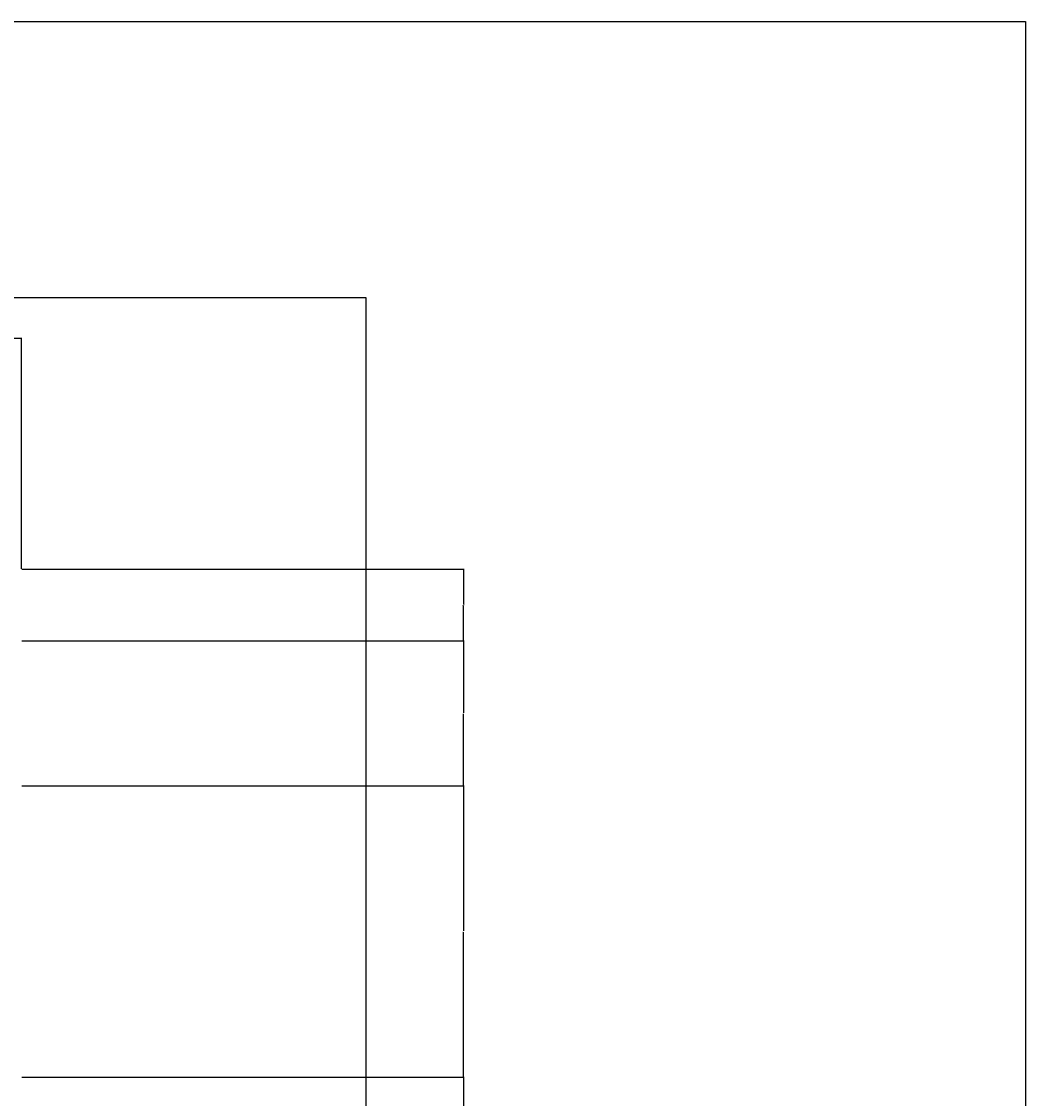
# Model space of a CAD drawing. Units: inches. Extents: x 1770 to 2988, y 1161 to 3221.
# Tile 44 of 44: x 2655 to 2988, y 2865 to 3221. Entities that reach past the tile are written whole.
import ezdxf

# ---------------------------------------------------------------- set-up
doc = ezdxf.new("R2010")
doc.units = ezdxf.units.IN
doc.layers.add('A-ANNO-DIMS', color=2, linetype='Continuous', lineweight=18)
doc.layers.add('A-ANNO-TTLB', color=7, linetype='Continuous', lineweight=25)
doc.styles.get("Standard").update_dxf_attribs({"font": 'arial.ttf'})
doc.dimstyles.get("Standard").update_dxf_attribs({"dimtxt": 0.18, "dimasz": 0.18, "dimexe": 0.18, "dimexo": 0.0625, "dimgap": 0.09, "dimtad": 0, "dimtih": 1, "dimtoh": 1, "dimdec": 4, "dimzin": 0, "dimdsep": 46, "dimtxsty": 'Standard', "dimcen": 0.09, "dimadec": 0, "dimazin": 0, "dimtfac": 1, "dimtdec": 4, "dimtofl": 0, "dimtmove": 0, "dimatfit": 3, "dimfxl": 1, "dimtolj": 1, "dimtzin": 0, "dimarcsym": 0})

# ---------------------------------------------------------------- blocks, each defined once
blk = doc.blocks.new('*D99')
at = {"layer": 'A-ANNO-DIMS', "color": 0, "lineweight": -2, "transparency": 16777216}
for p, q in [((2655.51, 2871.79), (2801.91, 2871.79)), ((2801.73, 2871.61), (2801.73, 2857.23)), ((2801.73, 2842.48), (2801.73, 2856.86)), ((2655.51, 2842.3), (2801.91, 2842.3))]:
    blk.add_line(p, q, dxfattribs=at)
at = {"layer": 'A-ANNO-DIMS', "color": 0, "transparency": 16777216}
for points in [[(2801.7, 2871.61), (2801.76, 2871.61), (2801.73, 2871.79)], [(2801.7, 2842.48), (2801.76, 2842.48), (2801.73, 2842.3)]]:
    blk.add_solid(points, dxfattribs=at)
at = {"layer": 'Defpoints', "color": 0, "transparency": 16777216}
for p in [(2655.44, 2871.79), (2801.73, 2871.79), (2655.44, 2842.3)]:
    blk.add_point(p, dxfattribs=at)
at = {"layer": 'A-ANNO-DIMS', "color": 0, "transparency": 16777216, "insert": (2801.73, 2857.05), "char_height": 0.18, "attachment_point": 5}
blk.add_mtext('\\A1;29.5', dxfattribs=at)
blk = doc.blocks.new('*D100')
at = {"layer": 'A-ANNO-DIMS', "color": 0, "lineweight": -2, "transparency": 16777216}
for p, q in [((2655.51, 2968.3), (2801.91, 2968.3)), ((2801.73, 2968.12), (2801.73, 2920.23)), ((2801.73, 2871.97), (2801.73, 2919.86)), ((2655.51, 2871.79), (2801.91, 2871.79))]:
    blk.add_line(p, q, dxfattribs=at)
at = {"layer": 'A-ANNO-DIMS', "color": 0, "transparency": 16777216}
for points in [[(2801.7, 2968.12), (2801.76, 2968.12), (2801.73, 2968.3)], [(2801.7, 2871.97), (2801.76, 2871.97), (2801.73, 2871.79)]]:
    blk.add_solid(points, dxfattribs=at)
at = {"layer": 'Defpoints', "color": 0, "transparency": 16777216}
for p in [(2655.44, 2968.3), (2801.73, 2968.3), (2655.44, 2871.79)]:
    blk.add_point(p, dxfattribs=at)
at = {"layer": 'A-ANNO-DIMS', "color": 0, "transparency": 16777216, "insert": (2801.73, 2920.05), "char_height": 0.18, "attachment_point": 5}
blk.add_mtext('\\A1;96.5', dxfattribs=at)
blk = doc.blocks.new('*D101')
at = {"layer": 'A-ANNO-DIMS', "color": 0, "lineweight": -2, "transparency": 16777216}
for p, q in [((2655.51, 3016.3), (2801.91, 3016.3)), ((2801.73, 3016.12), (2801.73, 2992.48)), ((2801.73, 2968.48), (2801.73, 2992.11)), ((2655.51, 2968.3), (2801.91, 2968.3))]:
    blk.add_line(p, q, dxfattribs=at)
at = {"layer": 'A-ANNO-DIMS', "color": 0, "transparency": 16777216}
for points in [[(2801.7, 3016.12), (2801.76, 3016.12), (2801.73, 3016.3)], [(2801.7, 2968.48), (2801.76, 2968.48), (2801.73, 2968.3)]]:
    blk.add_solid(points, dxfattribs=at)
at = {"layer": 'Defpoints', "color": 0, "transparency": 16777216}
for p in [(2655.44, 3016.3), (2801.73, 3016.3), (2655.44, 2968.3)]:
    blk.add_point(p, dxfattribs=at)
at = {"layer": 'A-ANNO-DIMS', "color": 0, "transparency": 16777216, "insert": (2801.73, 2992.3), "char_height": 0.18, "attachment_point": 5}
blk.add_mtext('\\A1;48', dxfattribs=at)
blk = doc.blocks.new('*D102')
at = {"layer": 'A-ANNO-DIMS', "color": 0, "lineweight": -2, "transparency": 16777216}
for p, q in [((2655.51, 3040.02), (2801.91, 3040.02)), ((2801.73, 3039.84), (2801.73, 3028.34)), ((2801.73, 3016.48), (2801.73, 3027.98)), ((2655.51, 3016.3), (2801.91, 3016.3))]:
    blk.add_line(p, q, dxfattribs=at)
at = {"layer": 'A-ANNO-DIMS', "color": 0, "transparency": 16777216}
for points in [[(2801.7, 3039.84), (2801.76, 3039.84), (2801.73, 3040.02)], [(2801.7, 3016.48), (2801.76, 3016.48), (2801.73, 3016.3)]]:
    blk.add_solid(points, dxfattribs=at)
at = {"layer": 'Defpoints', "color": 0, "transparency": 16777216}
for p in [(2655.44, 3040.02), (2801.73, 3040.02), (2655.44, 3016.3)]:
    blk.add_point(p, dxfattribs=at)
at = {"layer": 'A-ANNO-DIMS', "color": 0, "transparency": 16777216, "insert": (2801.73, 3028.16), "char_height": 0.18, "attachment_point": 5}
blk.add_mtext('\\A1;23.723', dxfattribs=at)
blk = doc.blocks.new('*D109')
at = {"layer": 'A-ANNO-DIMS', "color": 0, "lineweight": -2, "transparency": 16777216}
for p, q in [((2602.49, 3040.08), (2602.49, 3116.56)), ((2602.67, 3116.38), (2628.57, 3116.38)), ((2655.26, 3116.38), (2629.36, 3116.38)), ((2655.44, 3040.08), (2655.44, 3116.56))]:
    blk.add_line(p, q, dxfattribs=at)
at = {"layer": 'A-ANNO-DIMS', "color": 0, "transparency": 16777216}
for points in [[(2602.67, 3116.41), (2602.67, 3116.35), (2602.49, 3116.38)], [(2655.26, 3116.41), (2655.26, 3116.35), (2655.44, 3116.38)]]:
    blk.add_solid(points, dxfattribs=at)
at = {"layer": 'Defpoints', "color": 0, "transparency": 16777216}
for p in [(2655.44, 3116.38), (2602.49, 3040.02), (2655.44, 3040.02)]:
    blk.add_point(p, dxfattribs=at)
at = {"layer": 'A-ANNO-DIMS', "color": 0, "transparency": 16777216, "insert": (2628.96, 3116.38), "char_height": 0.18, "attachment_point": 5}
blk.add_mtext('\\A1;52.96', dxfattribs=at)

msp = doc.modelspace()

# ---------------------------------------------------------------- linework, layer by layer
at = {"layer": 'A-ANNO-TTLB'}
for points in [[(1769.9155, 3221.2788), (2987.7567, 3221.2788), (2987.7567, 1161.1516), (1769.9155, 1161.1516)], [(2073.6202, 3129.9468), (2769.3644, 3129.9468), (2769.3644, 2546.8952), (2073.6202, 2546.8952)]]:
    msp.add_lwpolyline(points, close=True, dxfattribs=at)

# ---------------------------------------------------------------- dimensions: what is measured, and where the dimension line sits
at = {"layer": 'A-ANNO-DIMS'}
dim = msp.add_linear_dim(base=(2655.443, 3116.3817), p1=(2602.4869, 3040.0203), p2=(2655.443, 3040.0203), dimstyle='Standard', override={"dimdec": 2, "dimlfac": 1, "dimrnd": 0, "dimzin": 0, "dimdsep": 46, "dimlunit": 2}, dxfattribs=at)
dim.commit()
dim.dimension.update_dxf_attribs({"geometry": '*D109', "text_midpoint": (2628.9649, 3116.3817)})
for base, p1, p2, override, picture, middle in [((2801.7346, 3040.0203), (2655.443, 3016.2969), (2655.443, 3040.0203), {"dimdec": 3, "dimlfac": 1, "dimrnd": 0, "dimzin": 0, "dimdsep": 46, "dimlunit": 2}, '*D102', (2801.7346, 3028.1586)), ((2801.7346, 3016.2969), (2655.443, 2968.2969), (2655.443, 3016.2969), {"dimdec": 0, "dimlfac": 1, "dimrnd": 0, "dimzin": 0, "dimdsep": 46, "dimlunit": 2}, '*D101', (2801.7346, 2992.2969)), ((2801.7346, 2968.2969), (2655.443, 2871.7944), (2655.443, 2968.2969), {"dimdec": 1, "dimlfac": 1, "dimrnd": 0, "dimzin": 0, "dimdsep": 46, "dimlunit": 2}, '*D100', (2801.7346, 2920.0456)), ((2801.7346, 2871.7944), (2655.443, 2842.2969), (2655.443, 2871.7944), {"dimdec": 1, "dimlfac": 1, "dimrnd": 0, "dimzin": 0, "dimdsep": 46, "dimlunit": 2}, '*D99', (2801.7346, 2857.0456))]:
    dim = msp.add_linear_dim(base=base, p1=p1, p2=p2, angle=90, dimstyle='Standard', override=override, dxfattribs=at)
    dim.commit()
    dim.dimension.update_dxf_attribs({"geometry": picture, "text_midpoint": middle})

doc.saveas('drawing.dxf')
